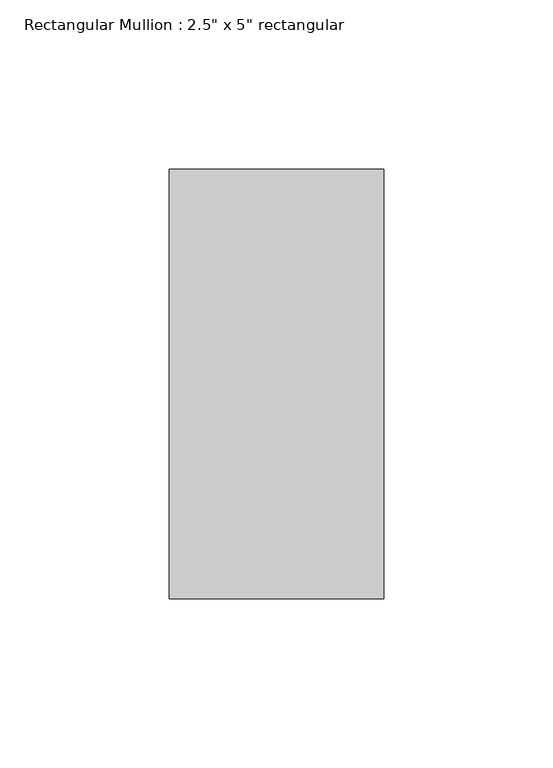
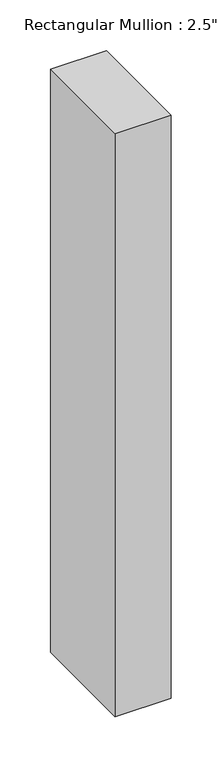
"""IFC4 building model written with IfcOpenShell, lengths in millimetres: member geometry."""

from ifc_helpers import new_model, si_unit, frame, origin, place, context, project, spatial, polyline, outline, extrude, source, transform, mapped, element, save


def member_3a8a164c(model_context):
    return source(origin(), model_context, "Body", "SweptSolid", [
        extrude(outline(polyline([(31.75, 63.5), (31.75, -63.5), (-31.75, -63.5), (-31.75, 63.5), (31.75, 63.5)])), frame((0.0, 0.0, -700.6166667), z_axis=(0.0, 0.0, 1.0), x_axis=(1.0, 0.0, 0.0)), (0.0, 0.0, 1.0), 700.6166667),
    ])


if __name__ == "__main__":
    model = new_model("IFC4")
    model_context = context("Model", 3, world=origin())
    ifc_project = project(units=[si_unit("LENGTHUNIT", "METRE", prefix="MILLI")], contexts=[model_context])
    site = spatial("IfcSite", under=ifc_project)
    building = spatial("IfcBuilding", under=site)
    placement = place(None, origin())
    member_shape = member_3a8a164c(model_context)
    element("IfcMember", 1, ObjectType="Rectangular Mullion : 2.5\" x 5\" rectangular", at=placement, inside=building, context=model_context, shape_type="MappedRepresentation", body=[
        mapped(member_shape, transform((0.0, 0.0, 0.0), x_axis=(1.0, 0.0, 0.0), y_axis=(0.0, 1.0, 0.0), z_axis=(0.0, 0.0, 1.0))),
    ])
    save(model, "model.ifc")

# Revit data of these elements
# Type "Rectangular Mullion : 2.5\" x 5\" rectangular"
#   built-in parameter 1007304 = 0.416667 (stored number, unit not read)
#   built-in parameter 1007301 = 0.104167 (stored number, unit not read)
#   built-in parameter 1007300 = 0.104167 (stored number, unit not read)
# Element 1 (IfcMember, "Rectangular Mullion : 2.5\" x 5\" rectangular")
#   Materials on its faces: "Aluminum"
# Materials
#   "Aluminum": class "Metal", colour RGB 247 247 247, transparency 0, Description = "Aluminum 6061", Cost = 0
